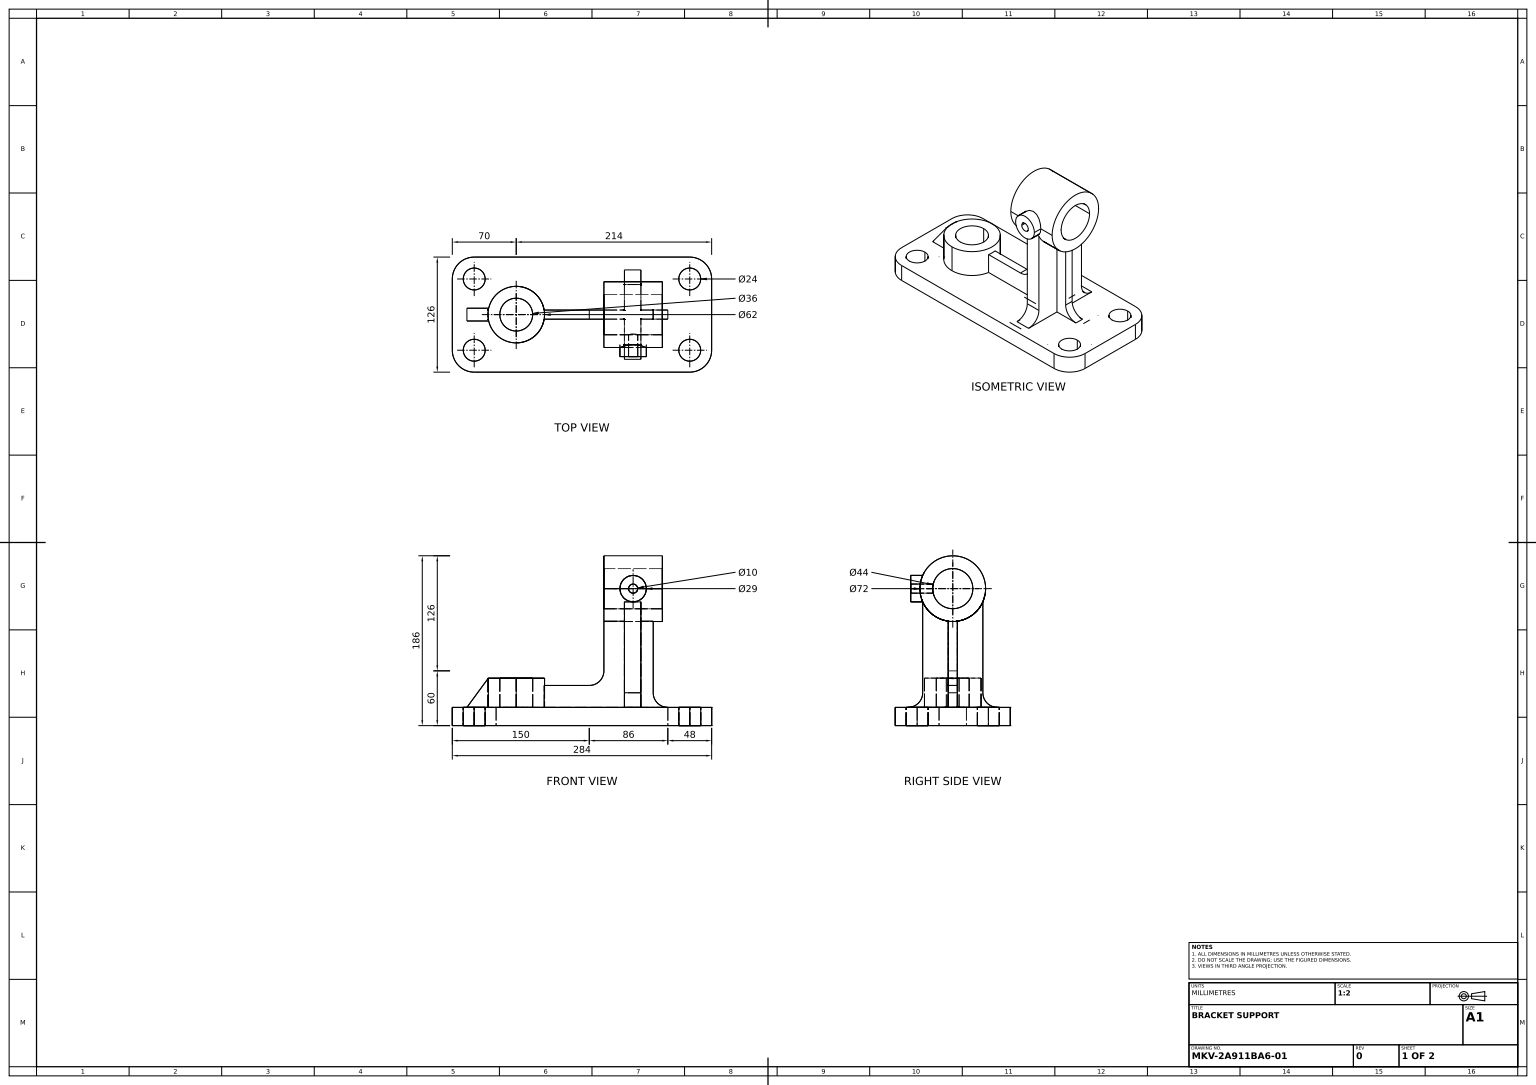
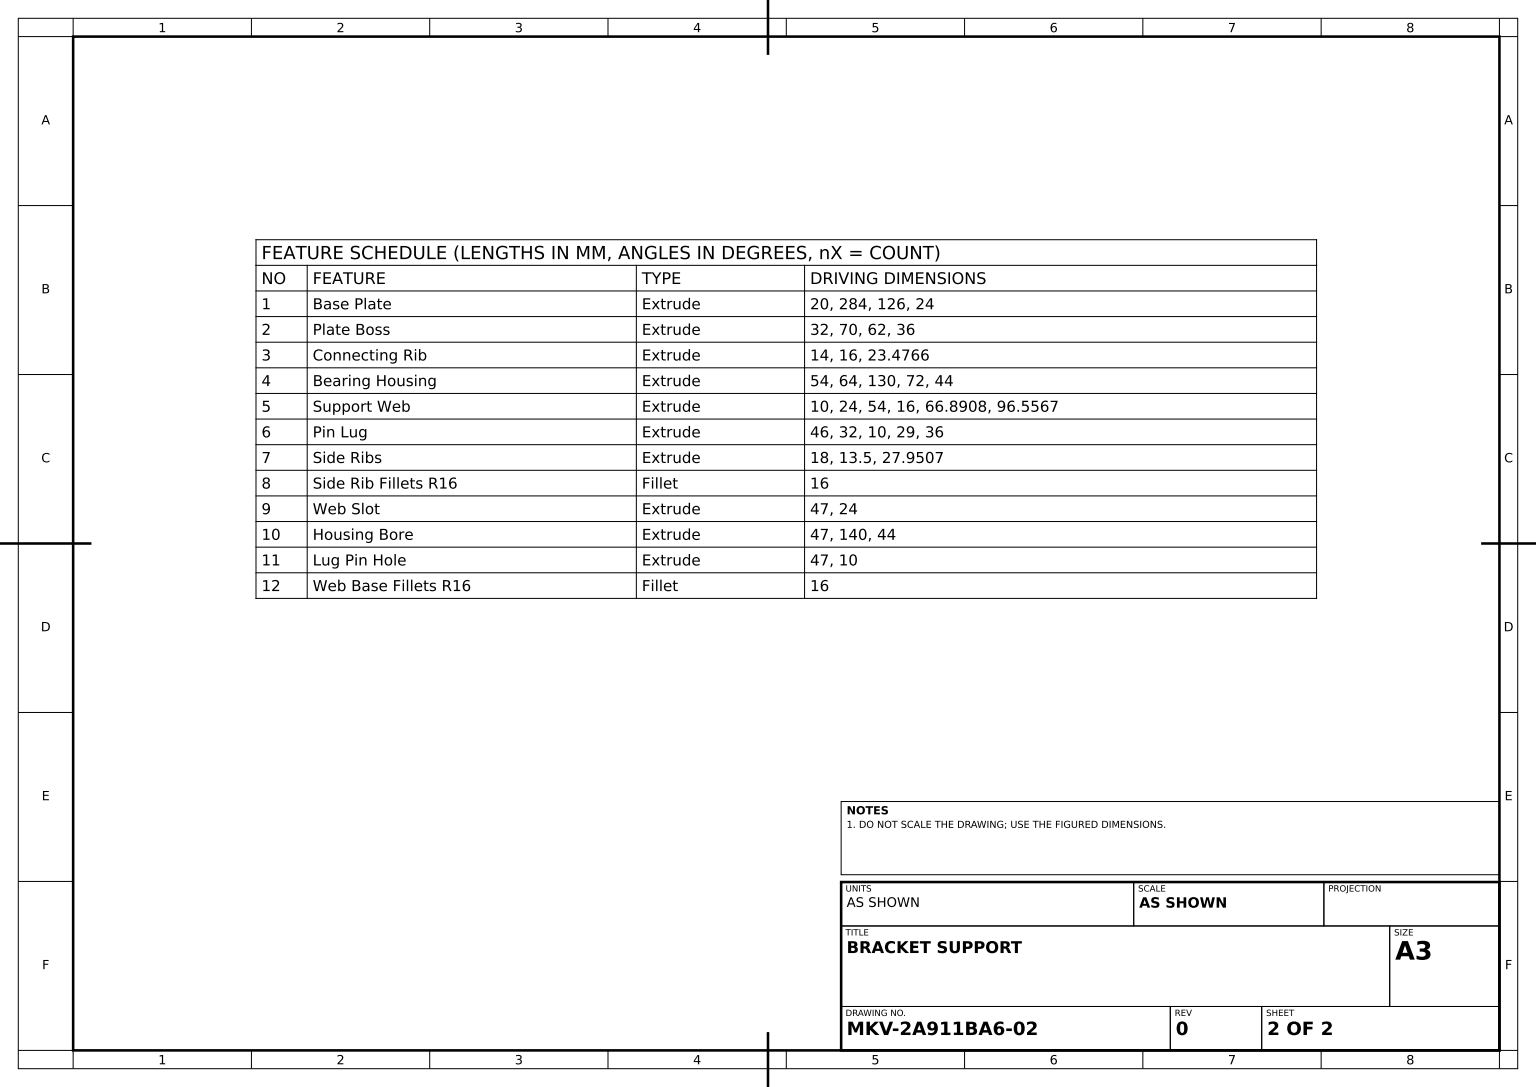
from build123d import *

# Parameters (mm, degrees)
BASE_PLATE_DEPTH           = 10
PLATE_BOSS_SKETCH_R        = 31
PLATE_BOSS_SKETCH_R_2      = 18
PLATE_BOSS_DEPTH           = 32
CONNECTING_RIB_DEPTH       = 7
BEARING_HOUSING_SKETCH_R   = 36
BEARING_HOUSING_SKETCH_R_2 = 22
BEARING_HOUSING_DEPTH      = 64
SUPPORT_WEB_DEPTH          = 5
PIN_LUG_SKETCH_R           = 14.5
PIN_LUG_SKETCH_R_2         = 5
PIN_LUG_DEPTH              = 46
SIDE_START                 = -13.5
SIDE_RIBS_DEPTH            = 18
SIDE_RIB_FILLETS_R16_R     = 16
WEB_SLOT_SKETCH_R          = 12
WEB_SLOT_DEPTH             = 47
HOUSING_BORE_SKETCH_R      = 22
HOUSING_BORE_DEPTH         = 47
LUG_START                  = -47
LUG_PIN_HOLE_SKETCH_R      = 5
LUG_PIN_HOLE_DEPTH         = 47
WEB_BASE_FILLETS_R16_R     = 16


with BuildPart() as part:
    # Base Plate Sketch → Base Plate (new, symmetric)
    with BuildSketch(Plane(origin=(0, 0, 0), x_dir=(1, 0, 0), z_dir=(0, 1, 0))):
        with BuildLine():
            Line((-118, 63), (118, 63))
            ThreePointArc((118, 63), (134.970562748, 55.970562748), (142, 39))
            Line((142, 39), (142, -39))
            ThreePointArc((142, -39), (134.970562748, -55.970562748), (118, -63))
            Line((118, -63), (-118, -63))
            ThreePointArc((-118, -63), (-134.970562748, -55.970562748), (-142, -39))
            Line((-142, -39), (-142, 39))
            ThreePointArc((-142, 39), (-134.970562748, 55.970562748), (-118, 63))
        make_face()
    extrude(amount=BASE_PLATE_DEPTH, both=True)

    # Plate Boss Sketch → Plate Boss (add)
    with BuildSketch(Plane(origin=(0, 10, 0), x_dir=(1, 0, 0), z_dir=(0, 1, 0))):
        with Locations(Location((-72, 0, 0), (0, 0, 270))):
            Circle(PLATE_BOSS_SKETCH_R)
        with Locations(Location((-72, 0, 0), (0, 0, 270))):
            Circle(PLATE_BOSS_SKETCH_R_2, mode=Mode.SUBTRACT)
    extrude(amount=PLATE_BOSS_DEPTH)

    # Connecting Rib Sketch → Connecting Rib (add, symmetric)
    with BuildSketch(Plane.XY):
        Polygon((-126, 10), (-102.523376003, 42), (-102.523376003, 10), align=None)
    extrude(amount=CONNECTING_RIB_DEPTH, both=True)



with BuildPart() as body_2:
    # Bearing Housing Sketch → Bearing Housing (new body)
    with BuildSketch(Plane(origin=(88, 0, 0), x_dir=(0, 0, -1), z_dir=(1, 0, 0))):
        with Locations((0, 140)):
            Circle(BEARING_HOUSING_SKETCH_R)
        with Locations((0, 140)):
            Circle(BEARING_HOUSING_SKETCH_R_2, mode=Mode.SUBTRACT)
    extrude(amount=-BEARING_HOUSING_DEPTH)


with BuildPart() as part_1:
    add(part.part)

    add(body_2.part)  # Support Web merges body 2
    # Support Web Sketch → Support Web (add, symmetric)
    with BuildSketch(Plane.XY):
        with BuildLine():
            Line((-42.890780427, 10), (-42.890780427, 34))
            Line((-42.890780427, 34), (8, 34))
            ThreePointArc((8, 34), (19.313708499, 38.686291501), (24, 50))
            Line((24, 50), (24, 106.55673196))
            Line((24, 106.55673196), (78, 106.55673196))
            Line((78, 106.55673196), (78, 10))
            Line((78, 10), (-42.890780427, 10))
        make_face()
    extrude(amount=SUPPORT_WEB_DEPTH, both=True)

    # Pin Lug Sketch → Pin Lug (add)
    with BuildSketch(Plane.XY):
        with Locations(Location((56, 140, 0), (0, 0, 180))):
            Circle(PIN_LUG_SKETCH_R)
        with Locations(Location((56, 140, 0), (0, 0, 180))):
            Circle(PIN_LUG_SKETCH_R_2, mode=Mode.SUBTRACT)
    extrude(amount=PIN_LUG_DEPTH)

    # Side Ribs Sketch → Side Ribs (add)
    with BuildSketch(Plane(origin=(78, 0, 0), x_dir=(0, 0, -1), z_dir=(1, 0, 0)).offset(SIDE_START)):
        with BuildLine():
            Line((-32.950720781, 125.5), (-32.950720781, 10))
            Line((-32.950720781, 10), (32.950720781, 10))
            Line((32.950720781, 10), (32.950720781, 125.5))
            ThreePointArc((32.950720781, 125.5), (0, 104), (-32.950720781, 125.5))
        make_face()
    extrude(amount=-SIDE_RIBS_DEPTH)

    # Side Rib Fillets R16
    side_rib_fillets_r16_edges = [part_1.edges().sort_by_distance(p)[0] for p in [
        (55.5, 10, -32.950720781),
        (55.5, 10, 32.950720781),
    ]]
    fillet(side_rib_fillets_r16_edges, radius=SIDE_RIB_FILLETS_R16_R)

    # Web Slot Sketch → Web Slot (cut)
    with BuildSketch(Plane(origin=(0, 10, 0), x_dir=(1, 0, 0), z_dir=(0, 1, 0))):
        with Locations(Location((-118, 39, 0), (0, 0, 270))):
            Circle(WEB_SLOT_SKETCH_R)
        with Locations(Location((-118, -39, 0), (0, 0, 270))):
            Circle(WEB_SLOT_SKETCH_R)
        with Locations(Location((118, -39, 0), (0, 0, 270))):
            Circle(WEB_SLOT_SKETCH_R)
        with Locations(Location((118, 39, 0), (0, 0, 270))):
            Circle(WEB_SLOT_SKETCH_R)
    extrude(amount=-WEB_SLOT_DEPTH, mode=Mode.SUBTRACT)

    # Housing Bore Sketch → Housing Bore (cut)
    with BuildSketch(Plane(origin=(88, 0, 0), x_dir=(0, 0, -1), z_dir=(1, 0, 0))):
        with Locations((0, 140)):
            Circle(HOUSING_BORE_SKETCH_R)
    extrude(amount=-HOUSING_BORE_DEPTH, mode=Mode.SUBTRACT)

    # Lug Pin Hole Sketch → Lug Pin Hole (cut)
    with BuildSketch(Plane.XY.offset(46).offset(LUG_START)):
        with Locations((56, 140)):
            Circle(LUG_PIN_HOLE_SKETCH_R)
    extrude(amount=LUG_PIN_HOLE_DEPTH, mode=Mode.SUBTRACT)

    # Web Base Fillets R16
    web_base_fillets_r16_edges = [part_1.edges().sort_by_distance(p)[0] for p in [
        (78, 10, 0),
    ]]
    fillet(web_base_fillets_r16_edges, radius=WEB_BASE_FILLETS_R16_R)


solid = part_1.part
